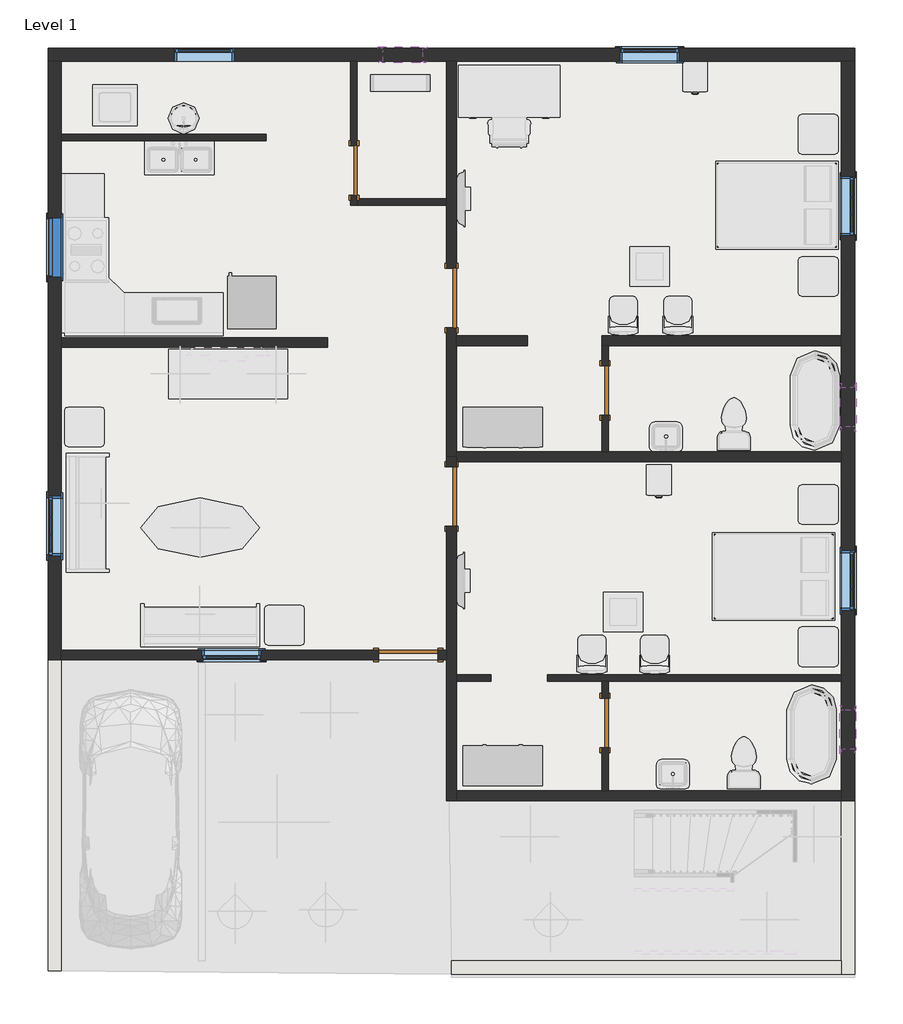
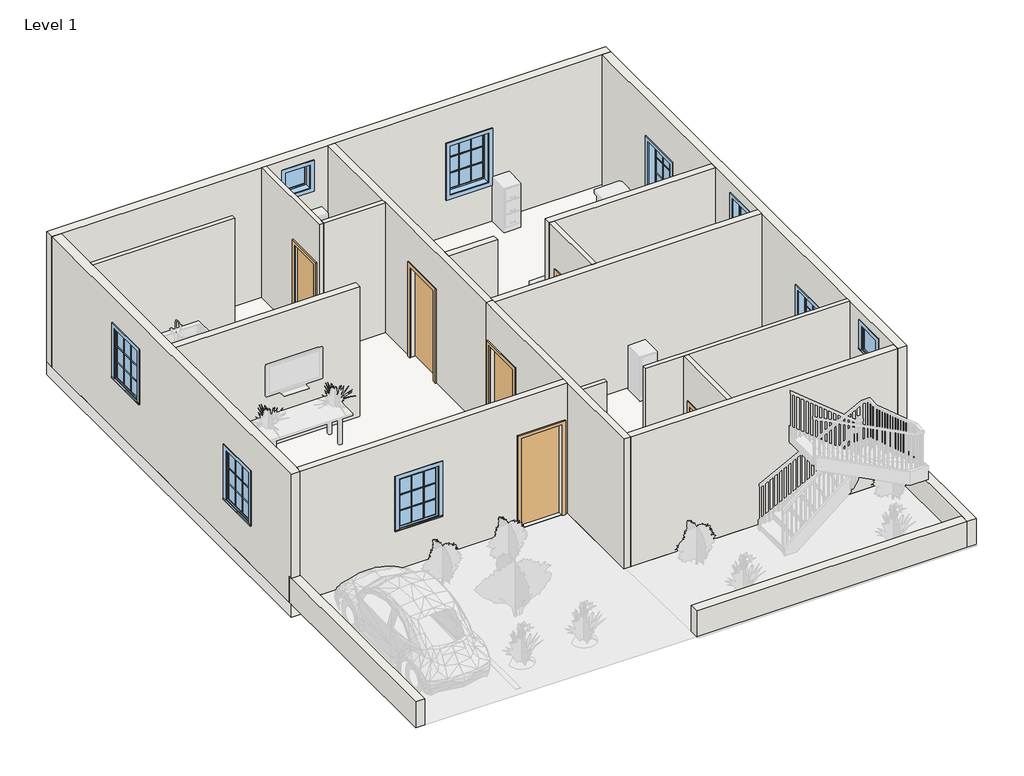
# One storey, part 1 of 3: 21 walls, 10 windows, 6 doors, 1 slab.
"""IFC4 building model written with IfcOpenShell, lengths in millimetres."""

from ifc_helpers import new_model, si_unit, frame, origin, origin_with_axes, place, context, project, spatial, polyline, outline, extrude, faceted_brep, transform, mapped, element, save
from components import door_29583826, door_98b18196, door_16372e1c, door_686f89d2, window_29c06734, window_5c190c7e, window_e2841890, window_e41d21a6

model = new_model("IFC4")

# Units and contexts
model_context = context("Model", 3, world=origin())
ifc_project = project(units=[si_unit("LENGTHUNIT", "METRE", prefix="MILLI")], contexts=[model_context])

# Site, building, storey
site = spatial("IfcSite", under=ifc_project)
building = spatial("IfcBuilding", under=site)
storey = spatial("IfcBuildingStorey", under=building, Name="Level 1", Elevation=0.0)

# Doors
placement = place(None, origin())
door_shape = door_29583826(model_context)
element("IfcDoor", 1, ObjectType="Single-Flush : 30\" x 80\"", at=placement, inside=storey, context=model_context, shape_type="MappedRepresentation", body=[
    mapped(door_shape, transform((-453.4621755, 6880.1807133, 0.0), x_axis=(0.0, -1.0, 0.0), y_axis=(1.0, 0.0, 0.0), z_axis=(0.0, 0.0, 1.0))),
])
door_2_shape = door_98b18196(model_context)
element("IfcDoor", 2, ObjectType="Single-Flush : 30\" x 80\"", at=placement, inside=storey, context=model_context, shape_type="MappedRepresentation", body=[
    mapped(door_2_shape, transform((3407.3378245, 3501.9807133, 0.0), x_axis=(0.0, 1.0, 0.0), y_axis=(-1.0, 0.0, 0.0), z_axis=(0.0, 0.0, 1.0))),
])
element("IfcDoor", 3, ObjectType="Single-Flush : 30\" x 80\"", at=placement, inside=storey, context=model_context, shape_type="MappedRepresentation", body=[
    mapped(door_2_shape, transform((3407.3378245, -1603.4192867, 0.0), x_axis=(0.0, 1.0, 0.0), y_axis=(-1.0, 0.0, 0.0), z_axis=(0.0, 0.0, 1.0))),
])
door_3_shape = door_16372e1c(model_context)
element("IfcDoor", 4, ObjectType="Single-Flush : 36\" x 84\"", at=placement, inside=storey, context=model_context, shape_type="MappedRepresentation", body=[
    mapped(door_3_shape, transform((384.7378245, -562.0192867, 0.0), x_axis=(1.0, 0.0, 0.0), y_axis=(0.0, 1.0, 0.0), z_axis=(0.0, 0.0, 1.0))),
])
element("IfcDoor", 5, ObjectType="Single-Flush : 36\" x 84\"", at=placement, inside=storey, context=model_context, shape_type="MappedRepresentation", body=[
    mapped(door_3_shape, transform((1045.1378245, 4924.3807133, 0.0), x_axis=(0.0, -1.0, 0.0), y_axis=(1.0, 0.0, 0.0), z_axis=(0.0, 0.0, 1.0))),
])
door_4_shape = door_686f89d2(model_context)
element("IfcDoor", 6, ObjectType="Single-Flush : 36\" x 84\"", at=placement, inside=storey, context=model_context, shape_type="MappedRepresentation", body=[
    mapped(door_4_shape, transform((1045.1378245, 1876.3807133, 0.0), x_axis=(0.0, 1.0, 0.0), y_axis=(-1.0, 0.0, 0.0), z_axis=(0.0, 0.0, 1.0))),
])

# Slab
element("IfcSlab", 7, ObjectType="Generic - 12\"", at=placement, inside=storey, context=model_context, shape_type="SweptSolid", body=[
    extrude(outline(polyline([(7242.7378245, 8759.7807133), (7242.7378245, -2797.2192867), (968.9378245, -2797.2192867), (968.9378245, -638.2192867), (-5152.4621755, -638.2192867), (-5152.4621755, 8759.7807133), (7242.7378245, 8759.7807133)])), frame((0.0, 0.0, -304.8), z_axis=(0.0, 0.0, 1.0), x_axis=(1.0, 0.0, 0.0)), (0.0, 0.0, 1.0), 304.8),
])

# Walls
element("IfcWall", 8, ObjectType="Generic - 2'", at=placement, inside=storey, context=model_context, shape_type="Brep", body=[
    faceted_brep([(-5152.4621755, -562.0192867, 0.0), (-5152.4621755, -5413.4192867, 0.0), (-5152.4621755, -5413.4192867, 609.6), (-5152.4621755, -562.0192867, 609.6), (-4949.2621755, -562.0192867, 0.0), (-4949.2621755, -562.0192867, 609.6), (-4949.2621755, -5413.4192867, 609.6), (-4949.2621755, -5413.4192867, 0.0), (-4949.2621755, -638.2192867, 0.0)], [[[0, 1, 2, 3]], [[4, 5, 6, 7, 8]], [[1, 0, 4, 8, 7]], [[2, 1, 7, 6]], [[3, 2, 6, 5]], [[0, 3, 5, 4]]]),
])
element("IfcWall", 9, ObjectType="Generic - 2'", at=placement, inside=storey, context=model_context, shape_type="Brep", body=[
    faceted_brep([(7039.5378245, -2721.0192867, 0.0), (7039.5378245, -2797.2192867, 0.0), (7039.5378245, -5261.0192867, 0.0), (7039.5378245, -5464.2192867, 0.0), (7039.5378245, -5464.2192867, 609.6), (7039.5378245, -5261.0192867, 609.6), (7039.5378245, -2721.0192867, 609.6), (7242.7378245, -2721.0192867, 0.0), (7242.7378245, -2721.0192867, 609.6), (7242.7378245, -5464.2192867, 609.6), (7242.7378245, -5464.2192867, 0.0)], [[[0, 1, 2, 3, 4, 5, 6]], [[7, 8, 9, 10]], [[3, 2, 1, 0, 7, 10]], [[6, 5, 4, 9, 8]], [[0, 6, 8, 7]], [[4, 3, 10, 9]]]),
])
element("IfcWall", 10, ObjectType="Generic - 2'", at=placement, inside=storey, context=model_context, shape_type="SweptSolid", body=[
    extrude(outline(polyline([(7039.5378245, -5464.2192867), (1045.1378245, -5464.2192867), (1045.1378245, -5261.0192867), (7039.5378245, -5261.0192867), (7039.5378245, -5464.2192867)])), origin_with_axes(), (0.0, 0.0, 1.0), 609.6),
])
element("IfcWall", 11, ObjectType="Generic - 8\"", at=placement, inside=storey, context=model_context, shape_type="Brep", body=[
    faceted_brep([(-5152.4621755, 8556.5807133, 0.0), (-4949.2621755, 8556.5807133, 0.0), (-504.2621755, 8556.5807133, 0.0), (-402.6621755, 8556.5807133, 0.0), (968.9378245, 8556.5807133, 0.0), (1121.3378245, 8556.5807133, 0.0), (7039.5378245, 8556.5807133, 0.0), (7242.7378245, 8556.5807133, 0.0), (7242.7378245, 8556.5807133, 3048.0), (7039.5378245, 8556.5807133, 3048.0), (1121.3378245, 8556.5807133, 3048.0), (968.9378245, 8556.5807133, 3048.0), (-402.6621755, 8556.5807133, 3048.0), (-504.2621755, 8556.5807133, 3048.0), (-4949.2621755, 8556.5807133, 3048.0), (-5152.4621755, 8556.5807133, 3048.0), (-2294.9621755, 8556.5807133, 2133.6), (-2294.9621755, 8556.5807133, 914.4), (-3209.3621755, 8556.5807133, 914.4), (-3209.3621755, 8556.5807133, 2133.6), (4550.3378245, 8556.5807133, 2133.6), (4550.3378245, 8556.5807133, 914.4), (3635.9378245, 8556.5807133, 914.4), (3635.9378245, 8556.5807133, 2133.6), (600.6378245, 8556.5807133, 2768.6), (600.6378245, 8556.5807133, 2159.0), (-8.9621755, 8556.5807133, 2159.0), (-8.9621755, 8556.5807133, 2768.6), (-5152.4621755, 8759.7807133, 0.0), (-5152.4621755, 8759.7807133, 3048.0), (7242.7378245, 8759.7807133, 3048.0), (7242.7378245, 8759.7807133, 0.0), (-2294.9621755, 8759.7807133, 2133.6), (-3209.3621755, 8759.7807133, 2133.6), (-3209.3621755, 8759.7807133, 914.4), (-2294.9621755, 8759.7807133, 914.4), (4550.3378245, 8759.7807133, 2133.6), (3635.9378245, 8759.7807133, 2133.6), (3635.9378245, 8759.7807133, 914.4), (4550.3378245, 8759.7807133, 914.4), (600.6378245, 8759.7807133, 2768.6), (-8.9621755, 8759.7807133, 2768.6), (-8.9621755, 8759.7807133, 2159.0), (600.6378245, 8759.7807133, 2159.0)], [[[0, 1, 2, 3, 4, 5, 6, 7, 8, 9, 10, 11, 12, 13, 14, 15], [16, 17, 18, 19], [20, 21, 22, 23], [24, 25, 26, 27]], [[28, 29, 30, 31], [32, 33, 34, 35], [36, 37, 38, 39], [40, 41, 42, 43]], [[7, 6, 5, 4, 3, 2, 1, 0, 28, 31]], [[8, 7, 31, 30]], [[0, 15, 29, 28]], [[17, 16, 32, 35]], [[18, 17, 35, 34]], [[19, 18, 34, 33]], [[16, 19, 33, 32]], [[21, 20, 36, 39]], [[22, 21, 39, 38]], [[23, 22, 38, 37]], [[20, 23, 37, 36]], [[25, 24, 40, 43]], [[26, 25, 43, 42]], [[27, 26, 42, 41]], [[24, 27, 41, 40]], [[15, 14, 13, 12, 11, 10, 9, 8, 30, 29]]]),
])
element("IfcWall", 12, ObjectType="Generic - 8\"", at=placement, inside=storey, context=model_context, shape_type="Brep", body=[
    faceted_brep([(7039.5378245, 8556.5807133, 0.0), (7039.5378245, 4340.1807133, 0.0), (7039.5378245, 4187.7807133, 0.0), (7039.5378245, 2562.1807133, 0.0), (7039.5378245, 2409.7807133, 0.0), (7039.5378245, -866.8192867, 0.0), (7039.5378245, -968.4192867, 0.0), (7039.5378245, -2644.8192867, 0.0), (7039.5378245, -2721.0192867, 0.0), (7039.5378245, -2721.0192867, 609.6), (7039.5378245, -2797.2192867, 609.6), (7039.5378245, -2797.2192867, 3048.0), (7039.5378245, -2644.8192867, 3048.0), (7039.5378245, -968.4192867, 3048.0), (7039.5378245, -866.8192867, 3048.0), (7039.5378245, 2409.7807133, 3048.0), (7039.5378245, 2562.1807133, 3048.0), (7039.5378245, 4187.7807133, 3048.0), (7039.5378245, 4340.1807133, 3048.0), (7039.5378245, 8556.5807133, 3048.0), (7039.5378245, 123.7807133, 2133.6), (7039.5378245, 123.7807133, 914.4), (7039.5378245, 1038.1807133, 914.4), (7039.5378245, 1038.1807133, 2133.6), (7039.5378245, 5876.8807133, 2133.6), (7039.5378245, 5876.8807133, 914.4), (7039.5378245, 6791.2807133, 914.4), (7039.5378245, 6791.2807133, 2133.6), (7039.5378245, 2943.1807133, 2768.6), (7039.5378245, 2943.1807133, 2159.0), (7039.5378245, 3552.7807133, 2159.0), (7039.5378245, 3552.7807133, 2768.6), (7039.5378245, -1400.2192867, 2768.6), (7039.5378245, -2009.8192867, 2768.6), (7039.5378245, -2009.8192867, 2159.0), (7039.5378245, -1400.2192867, 2159.0), (7242.7378245, 8556.5807133, 0.0), (7242.7378245, 8556.5807133, 3048.0), (7242.7378245, -2797.2192867, 3048.0), (7242.7378245, -2797.2192867, 609.6), (7242.7378245, -2721.0192867, 609.6), (7242.7378245, -2721.0192867, 0.0), (7242.7378245, 123.7807133, 2133.6), (7242.7378245, 1038.1807133, 2133.6), (7242.7378245, 1038.1807133, 914.4), (7242.7378245, 123.7807133, 914.4), (7242.7378245, 5876.8807133, 2133.6), (7242.7378245, 6791.2807133, 2133.6), (7242.7378245, 6791.2807133, 914.4), (7242.7378245, 5876.8807133, 914.4), (7242.7378245, 2943.1807133, 2768.6), (7242.7378245, 3552.7807133, 2768.6), (7242.7378245, 3552.7807133, 2159.0), (7242.7378245, 2943.1807133, 2159.0), (7242.7378245, -1400.2192867, 2768.6), (7242.7378245, -1400.2192867, 2159.0), (7242.7378245, -2009.8192867, 2159.0), (7242.7378245, -2009.8192867, 2768.6)], [[[0, 1, 2, 3, 4, 5, 6, 7, 8, 9, 10, 11, 12, 13, 14, 15, 16, 17, 18, 19], [20, 21, 22, 23], [24, 25, 26, 27], [28, 29, 30, 31], [32, 33, 34, 35]], [[36, 37, 38, 39, 40, 41], [42, 43, 44, 45], [46, 47, 48, 49], [50, 51, 52, 53], [54, 55, 56, 57]], [[8, 7, 6, 5, 4, 3, 2, 1, 0, 36, 41]], [[0, 19, 37, 36]], [[21, 20, 42, 45]], [[22, 21, 45, 44]], [[23, 22, 44, 43]], [[20, 23, 43, 42]], [[25, 24, 46, 49]], [[26, 25, 49, 48]], [[27, 26, 48, 47]], [[24, 27, 47, 46]], [[29, 28, 50, 53]], [[30, 29, 53, 52]], [[31, 30, 52, 51]], [[28, 31, 51, 50]], [[55, 54, 32, 35]], [[56, 55, 35, 34]], [[57, 56, 34, 33]], [[54, 57, 33, 32]], [[9, 8, 41, 40]], [[39, 10, 9, 40]], [[11, 10, 39, 38]], [[19, 18, 17, 16, 15, 14, 13, 12, 11, 38, 37]]]),
])
element("IfcWall", 13, ObjectType="Generic - 8\"", at=placement, inside=storey, context=model_context, shape_type="Brep", body=[
    faceted_brep([(-5152.4621755, 8556.5807133, 0.0), (-5152.4621755, -562.0192867, 0.0), (-5152.4621755, -562.0192867, 609.6), (-5152.4621755, -638.2192867, 609.6), (-5152.4621755, -638.2192867, 3048.0), (-5152.4621755, 8556.5807133, 3048.0), (-5152.4621755, 1876.3807133, 2133.6), (-5152.4621755, 961.9807133, 2133.6), (-5152.4621755, 961.9807133, 914.4), (-5152.4621755, 1876.3807133, 914.4), (-5152.4621755, 6156.2807133, 2387.6), (-5152.4621755, 5241.8807133, 2387.6), (-5152.4621755, 5241.8807133, 1168.4), (-5152.4621755, 6156.2807133, 1168.4), (-4949.2621755, 8556.5807133, 0.0), (-4949.2621755, 8556.5807133, 3048.0), (-4949.2621755, 7438.9807133, 3048.0), (-4949.2621755, 7337.3807133, 3048.0), (-4949.2621755, 4314.7807133, 3048.0), (-4949.2621755, 4162.3807133, 3048.0), (-4949.2621755, -485.8192867, 3048.0), (-4949.2621755, -638.2192867, 3048.0), (-4949.2621755, -638.2192867, 609.6), (-4949.2621755, -562.0192867, 609.6), (-4949.2621755, -562.0192867, 0.0), (-4949.2621755, -485.8192867, 0.0), (-4949.2621755, 4162.3807133, 0.0), (-4949.2621755, 4314.7807133, 0.0), (-4949.2621755, 7337.3807133, 0.0), (-4949.2621755, 7438.9807133, 0.0), (-4949.2621755, 1876.3807133, 2133.6), (-4949.2621755, 1876.3807133, 914.4), (-4949.2621755, 961.9807133, 914.4), (-4949.2621755, 961.9807133, 2133.6), (-4949.2621755, 6156.2807133, 2387.6), (-4949.2621755, 6156.2807133, 1168.4), (-4949.2621755, 5241.8807133, 1168.4), (-4949.2621755, 5241.8807133, 2387.6)], [[[0, 1, 2, 3, 4, 5], [6, 7, 8, 9], [10, 11, 12, 13]], [[14, 15, 16, 17, 18, 19, 20, 21, 22, 23, 24, 25, 26, 27, 28, 29], [30, 31, 32, 33], [34, 35, 36, 37]], [[1, 0, 14, 29, 28, 27, 26, 25, 24]], [[0, 5, 15, 14]], [[31, 30, 6, 9]], [[32, 31, 9, 8]], [[33, 32, 8, 7]], [[30, 33, 7, 6]], [[35, 34, 10, 13]], [[36, 35, 13, 12]], [[37, 36, 12, 11]], [[34, 37, 11, 10]], [[2, 1, 24, 23]], [[22, 3, 2, 23]], [[4, 3, 22, 21]], [[5, 4, 21, 20, 19, 18, 17, 16, 15]]]),
])
element("IfcWall", 14, ObjectType="INNER WALL 4\"", at=placement, inside=storey, context=model_context, shape_type="Brep", body=[
    faceted_brep([(-504.2621755, 6499.1807133, 2032.0), (-504.2621755, 6499.1807133, 0.0), (-504.2621755, 6346.7807133, 0.0), (-504.2621755, 6346.7807133, 3048.0), (-504.2621755, 8556.5807133, 3048.0), (-504.2621755, 8556.5807133, 0.0), (-504.2621755, 7261.1807133, 0.0), (-504.2621755, 7261.1807133, 2032.0), (-402.6621755, 6346.7807133, 0.0), (-402.6621755, 6448.3807133, 0.0), (-402.6621755, 6499.1807133, 0.0), (-402.6621755, 6499.1807133, 2032.0), (-402.6621755, 7261.1807133, 2032.0), (-402.6621755, 7261.1807133, 0.0), (-402.6621755, 8556.5807133, 0.0), (-402.6621755, 8556.5807133, 3048.0), (-402.6621755, 6448.3807133, 3048.0), (-402.6621755, 6346.7807133, 3048.0)], [[[0, 1, 2, 3, 4, 5, 6, 7]], [[8, 9, 10, 11, 12, 13, 14, 15, 16, 17]], [[6, 5, 14, 13]], [[2, 1, 10, 9, 8]], [[5, 4, 15, 14]], [[3, 2, 8, 17]], [[11, 10, 1, 0]], [[12, 11, 0, 7]], [[13, 12, 7, 6]], [[4, 3, 17, 16, 15]]]),
])
element("IfcWall", 15, ObjectType="INNER WALL 4\"", at=placement, inside=storey, context=model_context, shape_type="SweptSolid", body=[
    extrude(outline(polyline([(968.9378245, 6346.7807133), (-402.6621755, 6346.7807133), (-402.6621755, 6448.3807133), (968.9378245, 6448.3807133), (968.9378245, 6346.7807133)])), origin_with_axes(), (0.0, 0.0, 1.0), 3048.0),
])
element("IfcWall", 16, ObjectType="INNER WALL 4\"", at=placement, inside=storey, context=model_context, shape_type="SweptSolid", body=[
    extrude(outline(polyline([(-1799.6621755, 7337.3807133), (-4949.2621755, 7337.3807133), (-4949.2621755, 7438.9807133), (-1799.6621755, 7438.9807133), (-1799.6621755, 7337.3807133)])), origin_with_axes(), (0.0, 0.0, 1.0), 3048.0),
])
element("IfcWall", 17, ObjectType="INNER WALL 4\"", at=placement, inside=storey, context=model_context, shape_type="SweptSolid", body=[
    extrude(outline(polyline([(4187.7807133, 0.0), (3882.9807133, 0.0), (3882.9807133, 2032.0), (3120.9807133, 2032.0), (3120.9807133, 0.0), (2562.1807133, 0.0), (2562.1807133, 3048.0), (4187.7807133, 3048.0), (4187.7807133, 0.0)])), frame((3356.5378245, 0.0, 0.0), z_axis=(1.0, 0.0, 0.0), x_axis=(0.0, 1.0, 0.0)), (0.0, 0.0, 1.0), 101.6),
])
element("IfcWall", 18, ObjectType="INNER WALL 4\"", at=placement, inside=storey, context=model_context, shape_type="SweptSolid", body=[
    extrude(outline(polyline([(1654.7378245, -968.4192867), (1121.3378245, -968.4192867), (1121.3378245, -866.8192867), (1654.7378245, -866.8192867), (1654.7378245, -968.4192867)])), origin_with_axes(), (0.0, 0.0, 1.0), 3048.0),
])
element("IfcWall", 19, ObjectType="INNER WALL 4\"", at=placement, inside=storey, context=model_context, shape_type="SweptSolid", body=[
    extrude(outline(polyline([(-968.4192867, 0.0), (-1222.4192867, 0.0), (-1222.4192867, 2032.0), (-1984.4192867, 2032.0), (-1984.4192867, 0.0), (-2644.8192867, 0.0), (-2644.8192867, 3048.0), (-968.4192867, 3048.0), (-968.4192867, 0.0)])), frame((3356.5378245, 0.0, 0.0), z_axis=(1.0, 0.0, 0.0), x_axis=(0.0, 1.0, 0.0)), (0.0, 0.0, 1.0), 101.6),
])
element("IfcWall", 20, ObjectType="INNER WALL 4\"", at=placement, inside=storey, context=model_context, shape_type="Brep", body=[
    faceted_brep([(2518.3378245, -968.4192867, 0.0), (3356.5378245, -968.4192867, 0.0), (3458.1378245, -968.4192867, 0.0), (7039.5378245, -968.4192867, 0.0), (7039.5378245, -968.4192867, 3048.0), (3458.1378245, -968.4192867, 3048.0), (3356.5378245, -968.4192867, 3048.0), (2518.3378245, -968.4192867, 3048.0), (2518.3378245, -866.8192867, 0.0), (2518.3378245, -866.8192867, 3048.0), (7039.5378245, -866.8192867, 3048.0), (7039.5378245, -866.8192867, 0.0)], [[[0, 1, 2, 3, 4, 5, 6, 7]], [[8, 9, 10, 11]], [[3, 2, 1, 0, 8, 11]], [[0, 7, 9, 8]], [[4, 3, 11, 10]], [[7, 6, 5, 4, 10, 9]]]),
])
element("IfcWall", 21, ObjectType="INNER WALL 6\"", at=placement, inside=storey, context=model_context, shape_type="Brep", body=[
    faceted_brep([(968.9378245, 4467.1807133, 2133.6), (968.9378245, 4467.1807133, 0.0), (968.9378245, 2485.9807133, 0.0), (968.9378245, 2485.9807133, 3048.0), (968.9378245, 6346.7807133, 3048.0), (968.9378245, 6448.3807133, 3048.0), (968.9378245, 8556.5807133, 3048.0), (968.9378245, 8556.5807133, 0.0), (968.9378245, 6448.3807133, 0.0), (968.9378245, 6346.7807133, 0.0), (968.9378245, 5381.5807133, 0.0), (968.9378245, 5381.5807133, 2133.6), (1121.3378245, 2485.9807133, 0.0), (1121.3378245, 2562.1807133, 0.0), (1121.3378245, 4187.7807133, 0.0), (1121.3378245, 4340.1807133, 0.0), (1121.3378245, 4467.1807133, 0.0), (1121.3378245, 4467.1807133, 2133.6), (1121.3378245, 5381.5807133, 2133.6), (1121.3378245, 5381.5807133, 0.0), (1121.3378245, 8556.5807133, 0.0), (1121.3378245, 8556.5807133, 3048.0), (1121.3378245, 4340.1807133, 3048.0), (1121.3378245, 4187.7807133, 3048.0), (1121.3378245, 2562.1807133, 3048.0), (1121.3378245, 2485.9807133, 3048.0)], [[[0, 1, 2, 3, 4, 5, 6, 7, 8, 9, 10, 11]], [[12, 13, 14, 15, 16, 17, 18, 19, 20, 21, 22, 23, 24, 25]], [[2, 1, 16, 15, 14, 13, 12]], [[10, 9, 8, 7, 20, 19]], [[3, 2, 12, 25]], [[7, 6, 21, 20]], [[17, 16, 1, 0]], [[18, 17, 0, 11]], [[19, 18, 11, 10]], [[6, 5, 4, 3, 25, 24, 23, 22, 21]]]),
])
element("IfcWall", 22, ObjectType="INNER WALL 6\"", at=placement, inside=storey, context=model_context, shape_type="Brep", body=[
    faceted_brep([(968.9378245, -485.8192867, 0.0), (841.9378245, -485.8192867, 0.0), (841.9378245, -485.8192867, 2133.6), (-72.4621755, -485.8192867, 2133.6), (-72.4621755, -485.8192867, 0.0), (-4949.2621755, -485.8192867, 0.0), (-4949.2621755, -485.8192867, 3048.0), (968.9378245, -485.8192867, 3048.0), (-2790.2621755, -485.8192867, 2133.6), (-2790.2621755, -485.8192867, 914.4), (-1875.8621755, -485.8192867, 914.4), (-1875.8621755, -485.8192867, 2133.6), (841.9378245, -638.2192867, 2133.6), (841.9378245, -638.2192867, 0.0), (968.9378245, -638.2192867, 0.0), (968.9378245, -638.2192867, 3048.0), (-4949.2621755, -638.2192867, 3048.0), (-4949.2621755, -638.2192867, 609.6), (-4949.2621755, -638.2192867, 0.0), (-72.4621755, -638.2192867, 0.0), (-72.4621755, -638.2192867, 2133.6), (-2790.2621755, -638.2192867, 2133.6), (-1875.8621755, -638.2192867, 2133.6), (-1875.8621755, -638.2192867, 914.4), (-2790.2621755, -638.2192867, 914.4), (-4949.2621755, -562.0192867, 0.0)], [[[0, 1, 2, 3, 4, 5, 6, 7], [8, 9, 10, 11]], [[12, 13, 14, 15, 16, 17, 18, 19, 20], [21, 22, 23, 24]], [[19, 18, 25, 5, 4]], [[14, 13, 1, 0]], [[0, 7, 15, 14]], [[2, 1, 13, 12]], [[3, 2, 12, 20]], [[4, 3, 20, 19]], [[9, 8, 21, 24]], [[10, 9, 24, 23]], [[11, 10, 23, 22]], [[8, 11, 22, 21]], [[5, 25, 18, 17, 16, 6]], [[7, 6, 16, 15]]]),
])
element("IfcWall", 23, ObjectType="INNER WALL 6\"", at=placement, inside=storey, context=model_context, shape_type="Brep", body=[
    faceted_brep([(1121.3378245, 2409.7807133, 0.0), (7039.5378245, 2409.7807133, 0.0), (7039.5378245, 2409.7807133, 3048.0), (1121.3378245, 2409.7807133, 3048.0), (1121.3378245, 2562.1807133, 0.0), (1121.3378245, 2562.1807133, 3048.0), (3356.5378245, 2562.1807133, 3048.0), (3458.1378245, 2562.1807133, 3048.0), (7039.5378245, 2562.1807133, 3048.0), (7039.5378245, 2562.1807133, 0.0), (3458.1378245, 2562.1807133, 0.0), (3356.5378245, 2562.1807133, 0.0), (1121.3378245, 2485.9807133, 0.0), (1121.3378245, 2485.9807133, 3048.0)], [[[0, 1, 2, 3]], [[4, 5, 6, 7, 8, 9, 10, 11]], [[1, 0, 12, 4, 11, 10, 9]], [[2, 1, 9, 8]], [[0, 3, 13, 5, 4, 12]], [[3, 2, 8, 7, 6, 5, 13]]]),
])
element("IfcWall", 24, ObjectType="INNER WALL 6\"", at=placement, inside=storey, context=model_context, shape_type="Brep", body=[
    faceted_brep([(1121.3378245, -2797.2192867, 0.0), (7039.5378245, -2797.2192867, 0.0), (7039.5378245, -2797.2192867, 609.6), (7039.5378245, -2797.2192867, 3048.0), (1121.3378245, -2797.2192867, 3048.0), (1121.3378245, -2644.8192867, 0.0), (1121.3378245, -2644.8192867, 3048.0), (3356.5378245, -2644.8192867, 3048.0), (3458.1378245, -2644.8192867, 3048.0), (7039.5378245, -2644.8192867, 3048.0), (7039.5378245, -2644.8192867, 0.0), (3458.1378245, -2644.8192867, 0.0), (3356.5378245, -2644.8192867, 0.0), (7039.5378245, -2721.0192867, 0.0)], [[[0, 1, 2, 3, 4]], [[5, 6, 7, 8, 9, 10, 11, 12]], [[1, 0, 5, 12, 11, 10, 13]], [[0, 4, 6, 5]], [[1, 13, 10, 9, 3, 2]], [[4, 3, 9, 8, 7, 6]]]),
])
element("IfcWall", 25, ObjectType="INNER WALL 6\"", at=placement, inside=storey, context=model_context, shape_type="Brep", body=[
    faceted_brep([(968.9378245, 2485.9807133, 3048.0), (968.9378245, 2485.9807133, 0.0), (968.9378245, 2333.5807133, 0.0), (968.9378245, 2333.5807133, 2133.6), (968.9378245, 1419.1807133, 2133.6), (968.9378245, 1419.1807133, 0.0), (968.9378245, -485.8192867, 0.0), (968.9378245, -638.2192867, 0.0), (968.9378245, -2797.2192867, 0.0), (968.9378245, -2797.2192867, 3048.0), (968.9378245, -638.2192867, 3048.0), (968.9378245, -485.8192867, 3048.0), (1121.3378245, 2485.9807133, 3048.0), (1121.3378245, 2409.7807133, 3048.0), (1121.3378245, -866.8192867, 3048.0), (1121.3378245, -968.4192867, 3048.0), (1121.3378245, -2644.8192867, 3048.0), (1121.3378245, -2797.2192867, 3048.0), (1121.3378245, -2797.2192867, 0.0), (1121.3378245, -2644.8192867, 0.0), (1121.3378245, -968.4192867, 0.0), (1121.3378245, -866.8192867, 0.0), (1121.3378245, 1419.1807133, 0.0), (1121.3378245, 1419.1807133, 2133.6), (1121.3378245, 2333.5807133, 2133.6), (1121.3378245, 2333.5807133, 0.0), (1121.3378245, 2409.7807133, 0.0), (1121.3378245, 2485.9807133, 0.0)], [[[0, 1, 2, 3, 4, 5, 6, 7, 8, 9, 10, 11]], [[12, 13, 14, 15, 16, 17, 18, 19, 20, 21, 22, 23, 24, 25, 26, 27]], [[18, 8, 7, 6, 5, 22, 21, 20, 19]], [[1, 27, 26, 25, 2]], [[1, 0, 12, 27]], [[9, 8, 18, 17]], [[3, 24, 23, 4]], [[4, 23, 22, 5]], [[24, 3, 2, 25]], [[17, 16, 15, 14, 13, 12, 0, 11, 10, 9]]]),
])
element("IfcWall", 26, ObjectType="INNER WALL 6\"", at=placement, inside=storey, context=model_context, shape_type="SweptSolid", body=[
    extrude(outline(polyline([(-4949.2621755, 4314.7807133), (-859.8621755, 4314.7807133), (-859.8621755, 4162.3807133), (-4949.2621755, 4162.3807133), (-4949.2621755, 4314.7807133)])), origin_with_axes(), (0.0, 0.0, 1.0), 3048.0),
])
element("IfcWall", 27, ObjectType="INNER WALL 6\"", at=placement, inside=storey, context=model_context, shape_type="SweptSolid", body=[
    extrude(outline(polyline([(2213.5378245, 4187.7807133), (1121.3378245, 4187.7807133), (1121.3378245, 4340.1807133), (2213.5378245, 4340.1807133), (2213.5378245, 4187.7807133)])), origin_with_axes(), (0.0, 0.0, 1.0), 3048.0),
])
element("IfcWall", 28, ObjectType="INNER WALL 6\"", at=placement, inside=storey, context=model_context, shape_type="Brep", body=[
    faceted_brep([(3356.5378245, 4187.7807133, 0.0), (3458.1378245, 4187.7807133, 0.0), (7039.5378245, 4187.7807133, 0.0), (7039.5378245, 4187.7807133, 3048.0), (3458.1378245, 4187.7807133, 3048.0), (3356.5378245, 4187.7807133, 3048.0), (3356.5378245, 4340.1807133, 0.0), (3356.5378245, 4340.1807133, 3048.0), (7039.5378245, 4340.1807133, 3048.0), (7039.5378245, 4340.1807133, 0.0)], [[[0, 1, 2, 3, 4, 5]], [[6, 7, 8, 9]], [[2, 1, 0, 6, 9]], [[3, 2, 9, 8]], [[0, 5, 7, 6]], [[5, 4, 3, 8, 7]]]),
])

# Windows
window_shape = window_29c06734(model_context)
element("IfcWindow", 29, ObjectType="Casement 3x3 with Trim : 36\" x 48\"", at=placement, inside=storey, context=model_context, shape_type="MappedRepresentation", body=[
    mapped(window_shape, transform((-5050.8621755, 1419.1807133, 0.0), x_axis=(0.0, 1.0, 0.0), y_axis=(-1.0, 0.0, 0.0), z_axis=(0.0, 0.0, 1.0))),
])
element("IfcWindow", 30, ObjectType="Casement 3x3 with Trim : 36\" x 48\"", at=placement, inside=storey, context=model_context, shape_type="MappedRepresentation", body=[
    mapped(window_shape, transform((7141.1378245, 580.9807133, 0.0), x_axis=(0.0, -1.0, 0.0), y_axis=(1.0, 0.0, 0.0), z_axis=(0.0, 0.0, 1.0))),
])
element("IfcWindow", 31, ObjectType="Casement 3x3 with Trim : 36\" x 48\"", at=placement, inside=storey, context=model_context, shape_type="MappedRepresentation", body=[
    mapped(window_shape, transform((7141.1378245, 6334.0807133, 0.0), x_axis=(0.0, -1.0, 0.0), y_axis=(1.0, 0.0, 0.0), z_axis=(0.0, 0.0, 1.0))),
])
element("IfcWindow", 32, ObjectType="Casement 3x3 with Trim : 36\" x 48\"", at=placement, inside=storey, context=model_context, shape_type="MappedRepresentation", body=[
    mapped(window_shape, transform((4093.1378245, 8658.1807133, 0.0), x_axis=(1.0, 0.0, 0.0), y_axis=(0.0, 1.0, 0.0), z_axis=(0.0, 0.0, 1.0))),
])
element("IfcWindow", 33, ObjectType="Casement 3x3 with Trim : 36\" x 48\"", at=placement, inside=storey, context=model_context, shape_type="MappedRepresentation", body=[
    mapped(window_shape, transform((-5050.8621755, 5699.0807133, 254.0), x_axis=(0.0, 1.0, 0.0), y_axis=(-1.0, 0.0, 0.0), z_axis=(0.0, 0.0, 1.0))),
])
window_2_shape = window_5c190c7e(model_context)
element("IfcWindow", 34, ObjectType="Casement 3x3 with Trim : 36\" x 48\"", at=placement, inside=storey, context=model_context, shape_type="MappedRepresentation", body=[
    mapped(window_2_shape, transform((-2333.0621755, -562.0192867, 0.0), x_axis=(-1.0, 0.0, 0.0), y_axis=(0.0, -1.0, 0.0), z_axis=(0.0, 0.0, 1.0))),
])
window_3_shape = window_e2841890(model_context)
element("IfcWindow", 35, ObjectType="Fixed : 36\" x 48\"", at=placement, inside=storey, context=model_context, shape_type="MappedRepresentation", body=[
    mapped(window_3_shape, transform((-2714.0621755, 8658.1807133, 0.0), x_axis=(1.0, 0.0, 0.0), y_axis=(0.0, 1.0, 0.0), z_axis=(0.0, 0.0, 1.0))),
])
window_4_shape = window_e41d21a6(model_context)
element("IfcWindow", 36, ObjectType="Transom with Trim : 24\" x 24\"", at=placement, inside=storey, context=model_context, shape_type="MappedRepresentation", body=[
    mapped(window_4_shape, transform((333.9378245, 8658.1807133, 0.0), x_axis=(1.0, 0.0, 0.0), y_axis=(0.0, 1.0, 0.0), z_axis=(0.0, 0.0, 1.0))),
])
element("IfcWindow", 37, ObjectType="Transom with Trim : 24\" x 24\"", at=placement, inside=storey, context=model_context, shape_type="MappedRepresentation", body=[
    mapped(window_4_shape, transform((7141.1378245, 3209.8807133, 0.0), x_axis=(0.0, -1.0, 0.0), y_axis=(1.0, 0.0, 0.0), z_axis=(0.0, 0.0, 1.0))),
])
element("IfcWindow", 38, ObjectType="Transom with Trim : 24\" x 24\"", at=placement, inside=storey, context=model_context, shape_type="MappedRepresentation", body=[
    mapped(window_4_shape, transform((7141.1378245, -1666.9192867, 0.0), x_axis=(0.0, 1.0, 0.0), y_axis=(-1.0, 0.0, 0.0), z_axis=(0.0, 0.0, 1.0))),
])

save(model, "model.ifc")

# Revit data of these elements
# Type "Single-Flush : 30\" x 80\""
#   Type Mark = "5"
#   Construction Type Id = "MDOOR"
#   Assembly Code = "C1020"
#   Analytic Construction = "Metal"
#   Thickness = 0' - 2"
#   Heat Transfer Coefficient (U) = 0.651978 BTU/(h·ft²·°F)
#   Height = 6' - 8"
#   Trim Projection Ext = 0' - 1"
#   Trim Projection Int = 0' - 1"
#   Trim Width = 0' - 3"
#   Width = 2' - 6"
#   Define Thermal Properties by = 1
#   Door Material = Door - Panel
#   Frame Material = Door - Frame
#   Visual Light Transmittance = 0
#   Solar Heat Gain Coefficient = 0
#   Function = (empty or 0)
#   Wall Closure = (empty or 0)
# Type "Single-Flush : 36\" x 84\""
#   Type Mark = "1"
#   Construction Type Id = "MDOOR"
#   Assembly Code = "C1020"
#   Analytic Construction = "Metal"
#   Thickness = 0' - 2"
#   Heat Transfer Coefficient (U) = 0.651978 BTU/(h·ft²·°F)
#   Height = 7' - 0"
#   Trim Projection Ext = 0' - 1"
#   Trim Projection Int = 0' - 1"
#   Trim Width = 0' - 3"
#   Width = 3' - 0"
#   Define Thermal Properties by = 1
#   Door Material = Door - Panel
#   Frame Material = Door - Frame
#   Visual Light Transmittance = 0
#   Solar Heat Gain Coefficient = 0
#   Function = (empty or 0)
#   Wall Closure = (empty or 0)
# Type "Generic - 12\""
#   Assembly Code = "B1010"
#   Function = 0
#   Layers, outside or top first: 1' - 0" "Default Wall" (function 1)
# Type "Generic - 2'"
#   Assembly Code = "B2010"
#   Layers, outside or top first: 0' - 8" "Carpet (1)" (function 1)
# Type "Generic - 8\""
#   Assembly Code = "B2010"
#   Layers, outside or top first: 0' - 8" "Brick, Common" (function 1)
# Type "INNER WALL 4\""
#   Assembly Code = "B2010"
#   Layers, outside or top first: 0' - 4" "Brick, Common" (function 1)
# Type "INNER WALL 6\""
#   Assembly Code = "B2010"
#   Layers, outside or top first: 0' - 6" "Brick, Common" (function 1)
# Type "Casement 3x3 with Trim : 36\" x 48\""
#   Type Mark = "10"
#   Construction Type Id = "GSP4R"
#   Assembly Code = "B2020100"
#   Analytic Construction = "1/8 in Pilkington single glazing"
#   Visual Light Transmittance = 0.9
#   Solar Heat Gain Coefficient = 0.78
#   Heat Transfer Coefficient (U) = 0.6496 BTU/(h·ft²·°F)
#   Height = 4' - 0"
#   Default Sill Height = 3' - 0"
#   Trim Projection - Ext. = 0' - 0 1/2"
#   Trim Projection - Int. = 0' - 0 3/4"
#   Trim Width - Exterior = 0' - 3 1/2"
#   Trim Width - Interior = 0' - 3 1/2"
#   Width = 3' - 0"
#   Window Inset = 0' - 0 3/4"
#   Define Thermal Properties by = 1
#   Glass Pane Material = Glass
#   Sash Material = Sash
#   Trim Exterior Material = Trim
#   Trim Interior Material = Trim
#   Wall Closure = (empty or 0)
# Type "Fixed : 36\" x 48\""
#   Type Mark = "1"
#   Construction Type Id = "GSP4R"
#   Assembly Code = "B2020100"
#   Analytic Construction = "1/8 in Pilkington single glazing"
#   Visual Light Transmittance = 0.9
#   Solar Heat Gain Coefficient = 0.78
#   Heat Transfer Coefficient (U) = 0.6496 BTU/(h·ft²·°F)
#   Height = 4' - 0"
#   Default Sill Height = 3' - 0"
#   Width = 3' - 0"
#   Window Inset = 0' - 0 3/4"
#   Define Thermal Properties by = 1
#   Glass Pane Material = Glass
#   Sash Material = Sash
#   Wall Closure = (empty or 0)
# Type "Transom with Trim : 24\" x 24\""
#   Type Mark = "13"
#   Construction Type Id = "GSP4R"
#   Assembly Code = "B2020100"
#   Analytic Construction = "1/8 in Pilkington single glazing"
#   Visual Light Transmittance = 0.9
#   Solar Heat Gain Coefficient = 0.78
#   Heat Transfer Coefficient (U) = 0.6496 BTU/(h·ft²·°F)
#   Height = 2' - 0"
#   Default Sill Height = 7' - 1"
#   Trim Projection - Ext. = 0' - 0 1/2"
#   Trim Projection - Int. = 0' - 0 3/4"
#   Trim Width - Exterior = 0' - 3 1/2"
#   Trim Width - Interior = 0' - 3 1/2"
#   Width = 2' - 0"
#   Window Inset = 0' - 0 3/4"
#   Define Thermal Properties by = 1
#   Glass Pane Material = Glass
#   Sash Material = Sash
#   Trim Exterior Material = Trim
#   Trim Interior Material = Trim
#   Wall Closure = (empty or 0)
# Elements 1, 2, 3 (IfcDoor, "Single-Flush : 30\" x 80\"")
#   Phase Created = New Construction
#   Materials on its faces: "Door - Frame", "Door - Panel"
# Elements 4, 5, 6 (IfcDoor, "Single-Flush : 36\" x 84\"")
#   Phase Created = New Construction
#   Materials on its faces: "Door - Frame", "Door - Panel"
# Element 7 (IfcSlab, "Generic - 12\"")
#   Height Offset From Level = 0' - 0"
#   Phase Created = New Construction
#   Materials on its faces: "Default Wall"
# Elements 8, 9, 10 (IfcWall, "Generic - 2'")
#   Top Offset = 0' - 0"
#   Base Offset = 0' - 0"
#   Unconnected Height = 2' - 0"
#   wall height = 2' - 0"
#   Phase Created = New Construction
#   Base Constraint = Level 1
#   Materials on its faces: "Carpet (1)"
# Elements 11, 12, 13 (IfcWall, "Generic - 8\"")
#   Top Offset = 0' - 0"
#   Base Offset = 0' - 0"
#   Unconnected Height = 10' - 0"
#   wall height = 10' - 0"
#   Phase Created = New Construction
#   Base Constraint = Level 1
#   Materials on its faces: "Brick, Common"
# Elements 14, 15, 16, 17, 18, 19, 20 (IfcWall, "INNER WALL 4\"")
#   Top Offset = 0' - 0"
#   Base Offset = 0' - 0"
#   Unconnected Height = 10' - 0"
#   wall height = 10' - 0"
#   Phase Created = New Construction
#   Base Constraint = Level 1
#   Materials on its faces: "Brick, Common"
# Elements 21, 22, 23, 24, 25, 26, 27, 28 (IfcWall, "INNER WALL 6\"")
#   Top Offset = 0' - 0"
#   Base Offset = 0' - 0"
#   Unconnected Height = 10' - 0"
#   wall height = 10' - 0"
#   Phase Created = New Construction
#   Base Constraint = Level 1
#   Materials on its faces: "Brick, Common"
# Element 29 (IfcWindow, "Casement 3x3 with Trim : 36\" x 48\"")
#   Mark = "3"
#   Phase Created = New Construction
#   Materials on its faces: "Sash", "Glass", "Trim"
# Element 30 (IfcWindow, "Casement 3x3 with Trim : 36\" x 48\"")
#   Mark = "5"
#   Phase Created = New Construction
#   Materials on its faces: "Sash", "Glass", "Trim"
# Element 31 (IfcWindow, "Casement 3x3 with Trim : 36\" x 48\"")
#   Mark = "6"
#   Phase Created = New Construction
#   Materials on its faces: "Sash", "Glass", "Trim"
# Element 32 (IfcWindow, "Casement 3x3 with Trim : 36\" x 48\"")
#   Mark = "7"
#   Phase Created = New Construction
#   Materials on its faces: "Sash", "Glass", "Trim"
# Element 33 (IfcWindow, "Casement 3x3 with Trim : 36\" x 48\"")
#   Mark = "11"
#   Phase Created = New Construction
#   Materials on its faces: "Sash", "Glass", "Trim"
# Element 34 (IfcWindow, "Casement 3x3 with Trim : 36\" x 48\"")
#   Mark = "4"
#   Phase Created = New Construction
#   Materials on its faces: "Sash", "Glass", "Trim"
# Element 35 (IfcWindow, "Fixed : 36\" x 48\"")
#   Mark = "1"
#   Phase Created = New Construction
#   Materials on its faces: "Sash", "Glass"
# Element 36 (IfcWindow, "Transom with Trim : 24\" x 24\"")
#   Mark = "8"
#   Phase Created = New Construction
#   Materials on its faces: "Sash", "Trim", "Glass"
# Element 37 (IfcWindow, "Transom with Trim : 24\" x 24\"")
#   Mark = "9"
#   Phase Created = New Construction
#   Materials on its faces: "Sash", "Trim", "Glass"
# Element 38 (IfcWindow, "Transom with Trim : 24\" x 24\"")
#   Mark = "10"
#   Phase Created = New Construction
#   Materials on its faces: "Sash", "Trim", "Glass"
# Materials
#   "Door - Panel": class "Wood", colour RGB 210 159 95, transparency 0
#   "Door - Frame": colour RGB 118 70 51, transparency 0
#   "Default Wall": colour RGB 128 128 128, transparency 0
#   "Carpet (1)": class "Carpet", colour RGB 124 80 67, transparency 0, Description = "Interior finish"
#   "Brick, Common": class "Masonry", colour RGB 170 98 104, transparency 0, Description = "Common brick", Cost = 0
#   "Glass": class "Glass", colour RGB 0 128 192, transparency 0.75, Description = "Soda Lime Glass", Cost = 0
#   "Sash": class "Wood", colour RGB 224 178 126, transparency 0
#   "Trim": class "Wood", colour RGB 224 178 126, transparency 0
# Room at (-2202.329, 5806.317) mm, phase "New Construction", upper level "Level 1", upper offset 10' - 0", lower offset 0' - 0"
#   Number = "2"
#   Name = "KITCHEN"
# Room at (320.475, 7338.92) mm, phase "New Construction", upper level "Level 1", upper offset 10' - 0", lower offset 0' - 0"
#   Number = "3"
#   Name = "STORE"
# Room at (-2295.324, 1567.721) mm, phase "New Construction", upper level "Level 1", upper offset 10' - 0", lower offset 0' - 0"
#   Number = "4"
#   Name = "LIVING"
# Room at (5393.036, -2003.436) mm, phase "New Construction", upper level "Level 1", upper offset 10' - 0", lower offset 0' - 0"
#   Number = "5"
# Room at (2362.498, -2003.436) mm, phase "New Construction", upper level "Level 1", upper offset 10' - 0", lower offset 0' - 0"
#   Number = "6"
#   Name = "DRESSING"
# Room at (2149.275, 3212.601) mm, phase "New Construction", upper level "Level 1", upper offset 10' - 0", lower offset 0' - 0"
#   Number = "7"
#   Name = "DRESSING"
# Room at (5345.584, 3212.601) mm, phase "New Construction", upper level "Level 1", upper offset 10' - 0", lower offset 0' - 0"
#   Number = "8"
# Room at (3984.17, 6076.764) mm, phase "New Construction", upper level "Level 1", upper offset 10' - 0", lower offset 0' - 0"
#   Number = "9"
#   Name = "BEDROOM"
# Room at (-3024.578, 7885.516) mm, phase "New Construction", upper level "Level 1", upper offset 10' - 0", lower offset 0' - 0"
#   Number = "1"
#   Name = "UTILITY"
